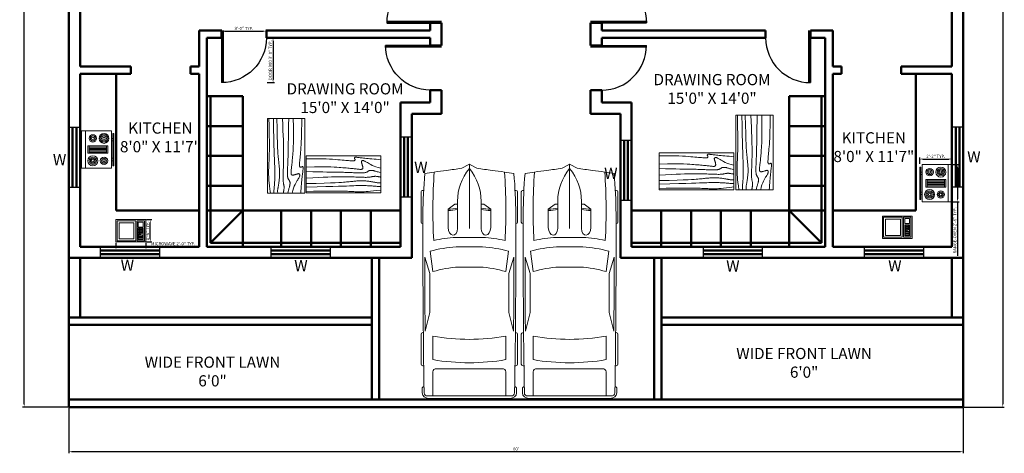
# Model space of a CAD drawing. Units: inches. Extents: x 2663 to 4539, y 2314 to 3111.
# Tile 1 of 4: x 2663 to 3456, y 2314 to 2663. Entities that reach past the tile are written whole.
import ezdxf

# ---------------------------------------------------------------- set-up
doc = ezdxf.new("R2010")
doc.units = ezdxf.units.IN
for name, color, linetype, lineweight in [('A-ANNO-DIMS', 2, 'Continuous', 18), ('A-ANNO-TEXT', 7, 'Continuous', 18), ('A-AREA-IDEN', 3, 'Continuous', 25), ('A-DOOR', 4, 'Continuous', 25), ('A-EQPM', 9, 'Continuous', 18), ('A-FURN', 8, 'Continuous', 18), ('A-GLAZ', 3, 'Continuous', 25), ('A-WALL', 7, 'Continuous', 50), ('C-PRKG', 9, 'Continuous', 18)]:
    doc.layers.add(name, color=color, linetype=linetype, lineweight=lineweight)
doc.styles.get("Standard").update_dxf_attribs({"font": 'arial.ttf'})
doc.dimstyles.new('ISO-25', dxfattribs={"dimtxt": 2.5, "dimasz": 2.5, "dimexe": 1.25, "dimexo": 0.625, "dimtad": 1, "dimdec": 0, "dimlunit": 3, "dimtxsty": 'Standard', "dimcen": 2.5, "dimadec": 0, "dimazin": 0, "dimtfac": 1, "dimtdec": 0, "dimtmove": 0, "dimatfit": 3, "dimfxl": 1, "dimarcsym": 0})

# ---------------------------------------------------------------- blocks, each defined once
blk = doc.blocks.new('Table - Rectangular Woodgrain 60 x 30 in.')
for p, q in [((0, 0), (0, -30)), ((60, 0), (0, 0)), ((60, -30), (60, 0)), ((0, -30), (60, -30))]:
    blk.add_line(p, q)
for points in [[(0, -2.4), (4.8155, -2.418), (9.0302, -2.4688), (12.709, -2.5477), (15.9167, -2.65), (18.7181, -2.7711), (21.1781, -2.9063), (23.3616, -3.0508), (25.3333, -3.2), (27.1477, -3.3495), (28.8172, -3.4958), (30.3437, -3.636), (31.7291, -3.7667), (32.9756, -3.8849), (34.0849, -3.9875), (35.059, -4.0714), (35.9, -4.1334), (36.6114, -4.1711), (37.2041, -4.1854), (37.6906, -4.1779), (38.0833, -4.15), (38.3948, -4.1034), (38.6375, -4.0396), (38.8239, -3.9602), (38.9666, -3.8667), (39.0764, -3.7608), (39.1573, -3.6448), (39.2116, -3.521), (39.2416, -3.3917), (39.2498, -3.2593), (39.2385, -3.1261), (39.21, -2.9944), (39.1666, -2.8667), (39.111, -2.7447), (39.0468, -2.6281), (38.978, -2.5163), (38.9083, -2.4083), (38.8418, -2.3035), (38.7823, -2.201), (38.7337, -2.1001), (38.7, -2), (38.6844, -1.9003), (38.6875, -1.8021), (38.7094, -1.707), (38.75, -1.6167), (38.8094, -1.5326), (38.8875, -1.4563), (38.9844, -1.3893), (39.1, -1.3333), (39.2351, -1.2896), (39.3937, -1.2583), (39.5804, -1.2396), (39.8, -1.2333), (40.057, -1.2396), (40.3562, -1.2583), (40.7023, -1.2896), (41.1, -1.3333), (41.5547, -1.3895), (42.0755, -1.4573), (42.6721, -1.5361), (43.3542, -1.625), (44.1316, -1.7233), (45.014, -1.8302), (46.0114, -1.9449), (47.1333, -2.0667), (48.3862, -2.1947), (49.7625, -2.3281), (51.2513, -2.4663), (52.8416, -2.6083), (54.5226, -2.7535), (56.2833, -2.9011), (58.1127, -3.0501), (60, -3.2)], [(0, -9.2), (6.5759, -9.0858), (11.9385, -9.0365), (16.2527, -9.0418), (19.6833, -9.0917), (22.3952, -9.1759), (24.5531, -9.2844), (26.322, -9.4069), (27.8666, -9.5333), (29.3241, -9.6553), (30.7203, -9.7719), (32.0532, -9.8837), (33.3208, -9.9917), (34.5213, -10.0965), (35.6526, -10.199), (36.7128, -10.2999), (37.7, -10.4), (38.6129, -10.4996), (39.4531, -10.5969), (40.223, -10.6895), (40.925, -10.775), (41.5613, -10.8512), (42.1344, -10.9156), (42.6465, -10.966), (43.1, -11), (43.4976, -11.0158), (43.8437, -11.0136), (44.143, -10.9942), (44.4, -10.9583), (44.6195, -10.9069), (44.8062, -10.8406), (44.9648, -10.7603), (45.1, -10.6667), (45.2155, -10.5598), (45.3114, -10.4365), (45.3871, -10.2929), (45.4416, -10.125), (45.4743, -9.929), (45.4844, -9.7011), (45.4709, -9.4371), (45.4333, -9.1333), (45.3716, -8.7883), (45.2896, -8.4104), (45.1919, -8.0107), (45.0833, -7.6), (44.9685, -7.1893), (44.8521, -6.7896), (44.7388, -6.4117), (44.6333, -6.0667), (44.54, -5.7628), (44.4614, -5.4979), (44.4001, -5.2675), (44.3583, -5.0667), (44.3384, -4.8909), (44.3427, -4.7354), (44.3736, -4.5956), (44.4333, -4.4667), (44.5236, -4.3453), (44.6427, -4.2333), (44.7884, -4.1339), (44.9583, -4.05), (45.1501, -3.9849), (45.3614, -3.9417), (45.59, -3.9234), (45.8333, -3.9333), (46.0915, -3.9749), (46.3734, -4.0531), (46.6906, -4.1736), (47.0542, -4.3417), (47.4756, -4.5629), (47.9661, -4.8427), (48.5372, -5.1866), (49.2, -5.6), (49.9676, -6.0844), (50.8594, -6.625), (51.8965, -7.2031), (53.1, -7.8), (54.491, -8.3969), (56.0906, -8.975), (57.9199, -9.5156), (60, -10)], [(0, -12.8), (5.1847, -12.9322), (9.6213, -13.0323), (13.3963, -13.1059), (16.5958, -13.1583), (19.3063, -13.1952), (21.614, -13.2219), (23.6054, -13.2439), (25.3666, -13.2667), (26.9728, -13.2947), (28.4531, -13.3281), (29.8256, -13.3663), (31.1083, -13.4083), (32.3191, -13.4535), (33.476, -13.501), (34.597, -13.5501), (35.7, -13.6), (36.7984, -13.6497), (37.8875, -13.6979), (38.9578, -13.743), (40, -13.7833), (41.0047, -13.8174), (41.9625, -13.8438), (42.864, -13.8607), (43.7, -13.8667), (44.4631, -13.8604), (45.1552, -13.8417), (45.7801, -13.8104), (46.3416, -13.7667), (46.8439, -13.7104), (47.2906, -13.6417), (47.6858, -13.5604), (48.0333, -13.4667), (48.3375, -13.3608), (48.6042, -13.2448), (48.8396, -13.121), (49.05, -12.9917), (49.2417, -12.8593), (49.4208, -12.7261), (49.5937, -12.5944), (49.7667, -12.4667), (49.9452, -12.3451), (50.1323, -12.2313), (50.3303, -12.1268), (50.5416, -12.0333), (50.7686, -11.9524), (51.0135, -11.8854), (51.2788, -11.8341), (51.5666, -11.8), (51.8785, -11.7843), (52.2116, -11.7865), (52.562, -11.8059), (52.926, -11.8417), (53.2998, -11.8931), (53.6795, -11.9594), (54.0614, -12.0397), (54.4416, -12.1333), (54.8223, -12.2401), (55.2293, -12.3625), (55.6942, -12.5037), (56.2489, -12.6667), (56.9251, -12.8547), (57.7545, -13.0708), (58.7689, -13.3182), (60, -13.6)], [(0, -18), (5.124, -17.7273), (9.6609, -17.5057), (13.6705, -17.3303), (17.2125, -17.1958), (20.3467, -17.0973), (23.1328, -17.0297), (25.6307, -16.9878), (27.9, -16.9667), (29.9928, -16.9617), (31.9302, -16.9703), (33.7254, -16.9907), (35.3917, -17.0208), (36.9423, -17.0588), (38.3906, -17.1026), (39.7499, -17.1503), (41.0333, -17.2), (42.2519, -17.2496), (43.4073, -17.2969), (44.4986, -17.3395), (45.525, -17.375), (46.4858, -17.4012), (47.3802, -17.4156), (48.2074, -17.416), (48.9667, -17.4), (49.6583, -17.3662), (50.2872, -17.3167), (50.8595, -17.2547), (51.3812, -17.1833), (51.8584, -17.1057), (52.2971, -17.025), (52.7034, -16.9443), (53.0833, -16.8667), (53.443, -16.7951), (53.789, -16.7313), (54.128, -16.6768), (54.4666, -16.6334), (54.8115, -16.6024), (55.1693, -16.5854), (55.5465, -16.5841), (55.95, -16.6), (56.3828, -16.6337), (56.8346, -16.6823), (57.2915, -16.7418), (57.7396, -16.8084), (58.165, -16.878), (58.5539, -16.9469), (58.8924, -17.0111), (59.1666, -17.0667), (59.3679, -17.1107), (59.5078, -17.1438), (59.6032, -17.1675), (59.6708, -17.1833), (59.7275, -17.193), (59.7901, -17.1979), (59.8753, -17.1998), (60, -17.2)], [(0, -22.4), (8.0098, -22.2501), (14.4094, -22.1011), (19.4168, -21.9535), (23.25, -21.8083), (26.1269, -21.6663), (28.2656, -21.5281), (29.884, -21.3947), (31.2, -21.2667), (32.3967, -21.1448), (33.5172, -21.0292), (34.5697, -20.9198), (35.5625, -20.8167), (36.5037, -20.7198), (37.4015, -20.6292), (38.2642, -20.5448), (39.1, -20.4667), (39.9164, -20.3951), (40.7187, -20.3313), (41.5117, -20.2768), (42.3, -20.2333), (43.0883, -20.2024), (43.8812, -20.1854), (44.6836, -20.1841), (45.5, -20.2), (46.3328, -20.234), (47.1747, -20.2844), (48.0163, -20.3488), (48.8479, -20.425), (49.66, -20.5106), (50.4429, -20.6031), (51.1872, -20.7004), (51.8833, -20.8), (52.5246, -20.8999), (53.1166, -20.9995), (53.6681, -21.0983), (54.1875, -21.1958), (54.6834, -21.2919), (55.1646, -21.3859), (55.6394, -21.4777), (56.1167, -21.5667), (56.6028, -21.6515), (57.0961, -21.7266), (57.5929, -21.7852), (58.0896, -21.8208), (58.5823, -21.8268), (59.0674, -21.7964), (59.5412, -21.723), (60, -21.6)], [(0, -25.2), (8.6355, -25.0504), (15.7026, -24.9031), (21.4049, -24.7606), (25.9458, -24.625), (29.529, -24.4988), (32.3578, -24.3844), (34.6359, -24.284), (36.5667, -24.2), (38.3213, -24.1341), (39.9417, -24.0854), (41.437, -24.0523), (42.8167, -24.0333), (44.0901, -24.0268), (45.2667, -24.0313), (46.3557, -24.0451), (47.3667, -24.0667), (48.309, -24.0947), (49.1928, -24.1287), (50.0284, -24.168), (50.826, -24.2125), (51.5959, -24.2617), (52.3483, -24.3151), (53.0935, -24.3725), (53.8417, -24.4334), (54.6009, -24.497), (55.3699, -24.561), (56.1454, -24.6226), (56.9239, -24.6792), (57.7021, -24.7279), (58.4764, -24.7662), (59.2435, -24.7911), (60, -24.8)], [(0, -28.8), (5.6867, -28.6681), (10.45, -28.5698), (14.407, -28.5012), (17.675, -28.4584), (20.3711, -28.4374), (22.6125, -28.4344), (24.5164, -28.4455), (26.2, -28.4667), (27.762, -28.4947), (29.2276, -28.5281), (30.6033, -28.5663), (31.8958, -28.6084), (33.1118, -28.6535), (34.2578, -28.7011), (35.3405, -28.7501), (36.3666, -28.8), (37.3443, -28.8497), (38.288, -28.8974), (39.2137, -28.9412), (40.1375, -28.9792), (41.0753, -29.0093), (42.0432, -29.0297), (43.0572, -29.0384), (44.1333, -29.0333), (45.2936, -29.0114), (46.5843, -28.9641), (48.0579, -28.8816), (49.7666, -28.7542), (51.7629, -28.5721), (54.0989, -28.3255), (56.8272, -28.0048), (60, -27.6)]]:
    blk.add_lwpolyline(points)
blk = doc.blocks.new('Range-Oven - 30 in top')
for p, q in [((0, -3), (30, -3)), ((12, -6), (18, -6)), ((13, -20), (13, -6)), ((14, -6), (14, -20)), ((15, -20), (15, -6)), ((16, -6), (16, -20)), ((17, -20), (17, -6)), ((18, -20), (12, -20)), ((6, -24), (6, -25)), ((8, -25), (8, -24)), ((22, -25), (22, -24)), ((24, -24), (24, -25))]:
    blk.add_line(p, q)
for points in [[(0, -24), (0, 0), (30, 0), (30, -24)], [(12, -21), (12, -5), (18, -5), (18, -21)], [(2, -26), (2, -25), (28, -25), (28, -26)]]:
    blk.add_lwpolyline(points, close=True)
for centre, radius in [((6, -9), 4), ((6, -9), 3), ((6, -9), 2), ((24, -9), 3), ((24, -9), 2), ((6, -18), 3), ((6, -9), 1), ((24, -18), 4), ((24, -18), 3), ((24, -9), 1), ((6, -18), 2), ((6, -18), 1), ((24, -18), 2), ((24, -18), 1)]:
    blk.add_circle(centre, radius)
blk = doc.blocks.new('Microwave')
for p, q in [((18, 10), (22, 10)), ((22, 9), (18, 9)), ((18, 8), (22, 8)), ((19, 7), (19, 11)), ((20, 11), (20, 7)), ((21, 7), (21, 11)), ((22, 7), (18, 7)), ((20, 6), (18, 6)), ((19, 6), (19, 7)), ((20, 7), (20, 6))]:
    blk.add_line(p, q)
for points in [[(0, 0), (0, 18), (24, 18), (24, 0)], [(1, 1), (1, 17), (16, 17), (16, 1)], [(17, 1), (17, 17), (23, 17), (23, 1)], [(18, 12), (18, 16), (22, 16), (22, 12)], [(2.5, 2.5), (2.5, 15.5), (14.5, 15.5), (14.5, 2.5)], [(18, 2), (18, 11), (22, 11), (22, 2)], [(18.5, 4.5), (18.5, 5.5), (21.5, 5.5), (21.5, 4.5)], [(18.5, 3), (18.5, 4), (21.5, 4), (21.5, 3)]]:
    blk.add_lwpolyline(points, close=True)
blk = doc.blocks.new('*D11')
at = {"layer": 'A-ANNO-DIMS', "color": 0, "lineweight": -2, "transparency": 16777216}
for p, q in [((3423.26, 3070.91), (3455.77, 3070.91)), ((3454.52, 3068.41), (3454.52, 2353.41)), ((3423.26, 2350.91), (3455.77, 2350.91))]:
    blk.add_line(p, q, dxfattribs=at)
at = {"layer": 'A-ANNO-DIMS', "color": 0, "transparency": 16777216}
for points in [[(3454.11, 3068.41), (3454.94, 3068.41), (3454.52, 3070.91)], [(3454.11, 2353.41), (3454.94, 2353.41), (3454.52, 2350.91)]]:
    blk.add_solid(points, dxfattribs=at)
at = {"layer": 'Defpoints', "color": 0, "transparency": 16777216}
for p in [(3422.63, 3070.91), (3422.63, 2350.91), (3454.52, 2350.91)]:
    blk.add_point(p, dxfattribs=at)
at = {"layer": 'A-ANNO-DIMS', "color": 0, "transparency": 16777216, "insert": (3452.62, 2710.91), "char_height": 2.5, "attachment_point": 5, "rotation": 90}
blk.add_mtext("60'", dxfattribs=at)
blk = doc.blocks.new('*U13')
for p, q in [((21.1, 37.41), (21.1, 36.83)), ((46.55, 38.89), (22.35, 38.89)), ((47.8, 37.39), (47.8, 37.41)), ((87.99, 31.87), (74.76, 35.92)), ((134.31, 35.6), (119.29, 31.78)), ((135.45, 37.07), (135.45, 37.41)), ((136.7, 38.89), (160.9, 38.89)), ((162.15, 37.41), (162.15, 36.77)), ((186.47, -33.5), (186.47, 33.5)), ((188.4, -32.76), (188.4, 32.76)), ((70.03, 31.54), (86.41, 29.35)), ((138.42, 29.35), (157.25, 29.35)), ((164.52, 26.39), (164.52, -26.39)), ((186.47, 29.35), (167.01, 29.35)), ((32.27, 11.63), (36.13, 17.17)), ((36.13, 17.17), (50.94, 17.17)), ((29.77, 9.51), (51.68, 9.51)), ((32.12, 9.51), (32.12, 11.15)), ((58.92, -10.77), (58.92, 10.77)), ((66.55, -10.53), (66.55, 10.53)), ((82.74, 8.5), (82.74, -8.5)), ((186.47, -10.53), (186.47, 10.53)), ((3.27, 6.13), (0.1, 0.41)), ((0, 0), (51.68, 0)), ((0.1, -0.41), (3.27, -6.13)), ((29.77, -9.51), (51.68, -9.51)), ((32.12, -9.51), (32.12, -11.15)), ((32.27, -11.63), (36.13, -17.17)), ((36.13, -17.17), (50.94, -17.17)), ((86.41, -29.35), (70.03, -31.54)), ((157.25, -29.35), (138.42, -29.35)), ((167.01, -29.35), (186.47, -29.35)), ((21.1, -37.41), (21.1, -36.83)), ((46.55, -38.89), (22.35, -38.89)), ((47.8, -37.39), (47.8, -37.41)), ((87.99, -31.87), (74.76, -35.92)), ((134.31, -35.6), (119.29, -31.78)), ((135.45, -37.07), (135.45, -37.41)), ((136.7, -38.89), (160.9, -38.89)), ((162.15, -37.41), (162.15, -36.77))]:
    blk.add_line(p, q)
for centre, major_axis, ratio, start_param, end_param in [((266.03, -27.52), (0, 313.31), 0.842304, 1.367076, 1.39176), ((41.19, -490.86), (0, 528.23), 0.842304, 0.00281, 0.075598), ((22.35, 37.41), (0, -1.48), 0.842304, 3.141593, 4.712389), ((64.48, -10555.62), (0, 10593.03), 0.842304, -0.013397, 0.002797), ((46.55, 37.41), (0, 1.48), 0.842304, -1.570796, 0), ((64.48, -10555.62), (0, -10591.55), 0.842304, 3.133765, 3.140441), ((95.79, -3666.35), (0, -3698.24), 0.842304, 3.134049, 3.144098), ((136.7, 37.41), (0, -1.48), 0.842304, 3.141593, 4.712389), ((160.9, 37.41), (0, 1.48), 0.842304, -1.570796, 0), ((180.63, 35.84), (0, 2.22), 0.842304, -0.013017, 1.249894), ((64.48, -10556.36), (0, 10595.31), 0.842304, -0.013397, -0.013017), ((183.98, 33.5), (0, -2.96), 0.842304, 1.570796, 3.128196), ((183.98, 32.76), (0, -5.25), 0.842304, 1.570796, 3.128196), ((259.18, -27.52), (0, -305.3), 0.842304, 4.528606, 4.561838), ((37.47, -593.96), (0, -623.33), 0.842304, 3.096046, 3.200911), ((134.4, 5.39), (0, -89.78), 0.842304, 4.449482, 4.652344), ((135.29, 5.39), (0, 81.77), 0.842304, 1.245306, 1.50788), ((149.6, 2.8), (0, -79.58), 0.842304, 4.372215, 4.640744), ((17.08, 0), (0, 147.02), 0.842304, 4.511394, 4.913384), ((35.91, 0), (0, 147.02), 0.842304, 4.511394, 4.913384), ((167.01, 26.39), (0, 2.96), 0.842304, 0, 1.570796), ((-204.49, 52.4), (0, -250.96), 0.842304, 1.385369, 1.434372), ((13.04, 17.01), (0, 27.42), 0.842304, 4.435146, 4.718221), ((14.2, 17.01), (0, 27.42), 0.842304, 4.435146, 4.718221), ((50.79, 13.34), (6.34, -0.36), 0.603834, -1.395552, 1.581315), ((29.77, -46.66), (0, 56.17), 0.842304, 0, 0.590319), ((32.75, 11.15), (0, 0.74), 0.842304, 0.879714, 1.570796), ((0.62, 0), (0, -0.74), 0.842304, 4.131459, 5.293319), ((-204.49, -52.4), (0, 250.96), 0.842304, -1.434372, -1.385369), ((29.77, 46.66), (0, 56.17), 0.842304, 2.551274, 3.141593), ((32.75, -11.15), (0, -0.74), 0.842304, 4.712389, 5.403472), ((13.04, -17.01), (0, -27.42), 0.842304, 1.564964, 1.848039), ((14.2, -17.01), (0, -27.42), 0.842304, 1.564964, 1.848039), ((134.4, -5.39), (0, -89.78), 0.842304, -1.510751, -1.307889), ((135.29, -5.39), (0, -81.77), 0.842304, -1.50788, -1.245306), ((149.6, -2.8), (0, -79.58), 0.842304, -1.499151, -1.230623), ((259.18, 27.52), (0, 305.3), 0.842304, 1.721348, 1.754579), ((266.03, 27.52), (0, 313.31), 0.842304, 1.749832, 1.774517), ((37.47, 593.96), (0, -623.33), 0.842304, -0.059319, 0.045547), ((167.01, -26.39), (0, -2.96), 0.842304, 4.712389, 6.283185), ((41.19, 490.86), (0, -528.23), 0.842304, -0.075598, -0.00281), ((22.35, -37.41), (0, 1.48), 0.842304, 1.570796, 3.141593), ((64.48, 10555.62), (0, 10593.03), 0.842304, 3.138796, 3.15499), ((46.55, -37.41), (0, -1.48), 0.842304, 0, 1.570796), ((64.48, 10555.62), (0, -10591.55), 0.842304, 0.001152, 0.007828), ((95.79, 3666.35), (0, -3698.24), 0.842304, -0.002505, 0.007544), ((136.7, -37.41), (0, -1.48), 0.842304, -1.570796, 0), ((160.9, -37.41), (0, 1.48), 0.842304, 3.141593, 4.712389), ((180.63, -35.84), (0, -2.22), 0.842304, -1.249894, 0.013017), ((64.48, 10556.36), (0, 10595.31), 0.842304, 3.15461, 3.15499), ((183.98, -33.5), (0, 2.96), 0.842304, 3.15499, 4.712389), ((183.98, -32.76), (0, -5.25), 0.842304, 0.013397, 1.570796)]:
    blk.add_ellipse(centre, major_axis=major_axis, ratio=ratio, start_param=start_param, end_param=end_param)
at = {"extrusion": (0, 0, -1)}
blk.add_ellipse((50.79, -13.34), major_axis=(6.34, 0.36), ratio=0.603834, start_param=-1.395552, end_param=1.581315, dxfattribs=at)
blk = doc.blocks.new('*D18')
at = {"layer": 'A-ANNO-DIMS', "color": 0, "lineweight": -2, "transparency": 16777216}
for p, q in [((2702.63, 2350.29), (2702.63, 2313.66)), ((3422.63, 2350.29), (3422.63, 2313.66)), ((3420.13, 2314.91), (2705.13, 2314.91))]:
    blk.add_line(p, q, dxfattribs=at)
at = {"layer": 'A-ANNO-DIMS', "color": 0, "transparency": 16777216}
for points in [[(2705.13, 2315.33), (2705.13, 2314.5), (2702.63, 2314.91)], [(3420.13, 2315.33), (3420.13, 2314.5), (3422.63, 2314.91)]]:
    blk.add_solid(points, dxfattribs=at)
at = {"layer": 'Defpoints', "color": 0, "transparency": 16777216}
for p in [(2702.63, 2350.91), (3422.63, 2350.91), (2702.63, 2314.91)]:
    blk.add_point(p, dxfattribs=at)
at = {"layer": 'A-ANNO-DIMS', "color": 0, "transparency": 16777216, "insert": (3062.63, 2316.82), "char_height": 2.5, "attachment_point": 5}
blk.add_mtext("60'", dxfattribs=at)
blk = doc.blocks.new('*D19')
at = {"layer": 'A-ANNO-DIMS', "color": 0, "lineweight": -2, "transparency": 16777216}
for p, q in [((2702.01, 3070.91), (2665.38, 3070.91)), ((2666.63, 2353.41), (2666.63, 3068.41)), ((2702.01, 2350.91), (2665.38, 2350.91))]:
    blk.add_line(p, q, dxfattribs=at)
at = {"layer": 'A-ANNO-DIMS', "color": 0, "transparency": 16777216}
for points in [[(2666.21, 3068.41), (2667.05, 3068.41), (2666.63, 3070.91)], [(2666.21, 2353.41), (2667.05, 2353.41), (2666.63, 2350.91)]]:
    blk.add_solid(points, dxfattribs=at)
at = {"layer": 'Defpoints', "color": 0, "transparency": 16777216}
for p in [(2666.63, 3070.91), (2702.63, 3070.91), (2702.63, 2350.91)]:
    blk.add_point(p, dxfattribs=at)
at = {"layer": 'A-ANNO-DIMS', "color": 0, "transparency": 16777216, "insert": (2664.73, 2710.91), "char_height": 2.5, "attachment_point": 5, "rotation": 90}
blk.add_mtext("60'", dxfattribs=at)
blk = doc.blocks.new('WIN-1200')
for p, q in [((0, 48), (0, 0)), ((9, 48), (0, 48)), ((0, 48), (0, 48)), ((9, 0), (9, 48)), ((0, 0), (9, 0))]:
    blk.add_line(p, q)
blk = doc.blocks.new('DOOR-900')
blk.add_line((3071.63, 2949.91), (3071.63, 2985.91))
blk.add_arc((3071.63, 2949.91), 36, 0, 90)
blk = doc.blocks.new('*D28')
at = {"layer": 'A-ANNO-DIMS', "color": 0, "lineweight": -2, "transparency": 16777216}
for p, q in [((2862.26, 2647.91), (2868.28, 2647.91)), ((2867.03, 2645.41), (2867.03, 2614.41)), ((2862.26, 2611.91), (2868.28, 2611.91))]:
    blk.add_line(p, q, dxfattribs=at)
at = {"layer": 'A-ANNO-DIMS', "color": 0, "transparency": 16777216}
for points in [[(2866.61, 2645.41), (2867.45, 2645.41), (2867.03, 2647.91)], [(2866.61, 2614.41), (2867.45, 2614.41), (2867.03, 2611.91)]]:
    blk.add_solid(points, dxfattribs=at)
at = {"layer": 'Defpoints', "color": 0, "transparency": 16777216}
for p in [(2861.63, 2647.91), (2861.63, 2611.91), (2867.03, 2611.91)]:
    blk.add_point(p, dxfattribs=at)
at = {"layer": 'A-ANNO-DIMS', "color": 0, "transparency": 16777216, "insert": (2865.11, 2629.91), "char_height": 2.5, "attachment_point": 5, "rotation": 90}
blk.add_mtext('DOOR 900 3\'-0" TYP.', dxfattribs=at)
blk = doc.blocks.new('*D29')
at = {"layer": 'A-ANNO-DIMS', "color": 0, "lineweight": -2, "transparency": 16777216}
for p, q in [((2825.63, 2648.54), (2825.63, 2654.56)), ((2828.13, 2653.31), (2859.13, 2653.31)), ((2861.63, 2648.54), (2861.63, 2654.56))]:
    blk.add_line(p, q, dxfattribs=at)
at = {"layer": 'A-ANNO-DIMS', "color": 0, "transparency": 16777216}
for points in [[(2828.13, 2653.73), (2828.13, 2652.9), (2825.63, 2653.31)], [(2859.13, 2653.73), (2859.13, 2652.9), (2861.63, 2653.31)]]:
    blk.add_solid(points, dxfattribs=at)
at = {"layer": 'Defpoints', "color": 0, "transparency": 16777216}
for p in [(2825.63, 2647.91), (2861.63, 2653.31), (2861.63, 2647.91)]:
    blk.add_point(p, dxfattribs=at)
at = {"layer": 'A-ANNO-DIMS', "color": 0, "transparency": 16777216, "insert": (2843.63, 2655.22), "char_height": 2.5, "attachment_point": 5}
blk.add_mtext('3\'-0" TYP.', dxfattribs=at)
blk = doc.blocks.new('*D46')
at = {"layer": 'A-ANNO-DIMS', "color": 0, "lineweight": -2, "transparency": 16777216}
for p, q in [((3414.26, 2545.91), (3419.38, 2545.91)), ((3418.13, 2543.41), (3418.13, 2518.41)), ((3414.26, 2515.91), (3419.38, 2515.91)), ((3418.13, 2515.91), (3418.13, 2472.6))]:
    blk.add_line(p, q, dxfattribs=at)
at = {"layer": 'A-ANNO-DIMS', "color": 0, "transparency": 16777216}
for points in [[(3417.71, 2543.41), (3418.55, 2543.41), (3418.13, 2545.91)], [(3417.71, 2518.41), (3418.55, 2518.41), (3418.13, 2515.91)]]:
    blk.add_solid(points, dxfattribs=at)
at = {"layer": 'Defpoints', "color": 0, "transparency": 16777216}
for p in [(3413.63, 2545.91), (3413.63, 2515.91), (3418.13, 2515.91)]:
    blk.add_point(p, dxfattribs=at)
at = {"layer": 'A-ANNO-DIMS', "color": 0, "transparency": 16777216, "insert": (3416.21, 2493), "char_height": 2.5, "attachment_point": 5, "rotation": 90}
blk.add_mtext('RANGE-OVEN 2\'-6" TYP.', dxfattribs=at)
blk = doc.blocks.new('*D47')
at = {"layer": 'A-ANNO-DIMS', "color": 0, "lineweight": -2, "transparency": 16777216}
for p, q in [((3387.63, 2546.53), (3387.63, 2551.66)), ((3390.13, 2550.41), (3411.13, 2550.41)), ((3413.63, 2546.53), (3413.63, 2551.66))]:
    blk.add_line(p, q, dxfattribs=at)
at = {"layer": 'A-ANNO-DIMS', "color": 0, "transparency": 16777216}
for points in [[(3390.13, 2550.82), (3390.13, 2549.99), (3387.63, 2550.41)], [(3411.13, 2550.82), (3411.13, 2549.99), (3413.63, 2550.41)]]:
    blk.add_solid(points, dxfattribs=at)
at = {"layer": 'Defpoints', "color": 0, "transparency": 16777216}
for p in [(3387.63, 2545.91), (3413.63, 2550.41), (3413.63, 2545.91)]:
    blk.add_point(p, dxfattribs=at)
at = {"layer": 'A-ANNO-DIMS', "color": 0, "transparency": 16777216, "insert": (3400.63, 2552.29), "char_height": 2.5, "attachment_point": 5}
blk.add_mtext('2\'-2" TYP.', dxfattribs=at)
blk = doc.blocks.new('*D48')
at = {"layer": 'A-ANNO-DIMS', "color": 0, "lineweight": -2, "transparency": 16777216}
for p, q in [((2740.52, 2483.06), (2740.52, 2478.84)), ((2764.52, 2483.06), (2764.52, 2478.84)), ((2743.02, 2480.09), (2762.02, 2480.09)), ((2764.52, 2480.09), (2806.29, 2480.09))]:
    blk.add_line(p, q, dxfattribs=at)
at = {"layer": 'A-ANNO-DIMS', "color": 0, "transparency": 16777216}
for points in [[(2743.02, 2480.51), (2743.02, 2479.67), (2740.52, 2480.09)], [(2762.02, 2480.51), (2762.02, 2479.67), (2764.52, 2480.09)]]:
    blk.add_solid(points, dxfattribs=at)
at = {"layer": 'Defpoints', "color": 0, "transparency": 16777216}
for p in [(2740.52, 2483.69), (2764.52, 2483.69), (2764.52, 2480.09)]:
    blk.add_point(p, dxfattribs=at)
at = {"layer": 'A-ANNO-DIMS', "color": 0, "transparency": 16777216, "insert": (2786.66, 2482.01), "char_height": 2.5, "attachment_point": 5}
blk.add_mtext('MICROWAVE 2\'-0" TYP.', dxfattribs=at)
blk = doc.blocks.new('*D49')
at = {"layer": 'A-ANNO-DIMS', "color": 0, "lineweight": -2, "transparency": 16777216}
for p, q in [((2765.15, 2501.69), (2769.37, 2501.69)), ((2768.12, 2486.19), (2768.12, 2499.19)), ((2765.15, 2483.69), (2769.37, 2483.69))]:
    blk.add_line(p, q, dxfattribs=at)
at = {"layer": 'A-ANNO-DIMS', "color": 0, "transparency": 16777216}
for points in [[(2767.7, 2499.19), (2768.54, 2499.19), (2768.12, 2501.69)], [(2767.7, 2486.19), (2768.54, 2486.19), (2768.12, 2483.69)]]:
    blk.add_solid(points, dxfattribs=at)
at = {"layer": 'Defpoints', "color": 0, "transparency": 16777216}
for p in [(2764.52, 2501.69), (2768.12, 2501.69), (2764.52, 2483.69)]:
    blk.add_point(p, dxfattribs=at)
at = {"layer": 'A-ANNO-DIMS', "color": 0, "transparency": 16777216, "insert": (2766.22, 2492.69), "char_height": 2.5, "attachment_point": 5, "rotation": 90}
blk.add_mtext('1\'-6" TYP.', dxfattribs=at)

msp = doc.modelspace()

# ---------------------------------------------------------------- linework, layer by layer
at = {"layer": 'A-DOOR'}
msp.add_arc((2993.63, 2660.91), 35, 90, 181.63725, dxfattribs=at)
at = {"layer": 'A-WALL'}
for p, q in [((2702.63, 2350.91), (2702.63, 3070.91)), ((3422.63, 3070.91), (3422.63, 2350.91)), ((2711.63, 2624.91), (2711.63, 3061.91)), ((3413.63, 2789.91), (3413.63, 2624.91)), ((2993.63, 2660.91), (2958.63, 2660.91)), ((2993.63, 2659.91), (2958.64, 2659.91)), ((2993.63, 2660.91), (3002.63, 2660.91)), ((2993.63, 2653.91), (2993.63, 2659.91)), ((2993.63, 2659.91), (3002.63, 2659.91)), ((2993.63, 2659.91), (2993.63, 2653.91)), ((3002.63, 2659.91), (3002.63, 2641.91)), ((3002.63, 2659.91), (3002.63, 2653.91)), ((3131.63, 2660.91), (3122.63, 2660.91)), ((3131.63, 2659.91), (3122.63, 2659.91)), ((3122.63, 2659.91), (3122.63, 2653.91)), ((3122.63, 2659.91), (3122.63, 2641.91)), ((3131.63, 2660.91), (3167.63, 2660.91)), ((3131.63, 2653.91), (3131.63, 2659.91)), ((3131.63, 2659.91), (3131.63, 2653.91)), ((2807.63, 2653.91), (2825.63, 2653.91)), ((2807.63, 2624.91), (2807.63, 2653.91)), ((2813.63, 2647.91), (2825.63, 2647.91)), ((2813.63, 2624.91), (2813.63, 2647.91)), ((2813.63, 2647.91), (2825.63, 2647.91)), ((2825.63, 2647.91), (2825.63, 2653.91)), ((2826.63, 2647.91), (2826.63, 2653.91)), ((2826.63, 2647.91), (2826.63, 2611.91)), ((2861.63, 2653.91), (2861.63, 2647.91)), ((2861.63, 2653.91), (2993.63, 2653.91)), ((2861.63, 2647.91), (2993.63, 2647.91)), ((2993.63, 2647.91), (2993.63, 2641.91)), ((2993.63, 2647.91), (2993.63, 2641.91)), ((3002.63, 2647.91), (3002.63, 2641.91)), ((3122.63, 2647.91), (3122.63, 2641.91)), ((3131.63, 2653.91), (3263.63, 2653.91)), ((3131.63, 2647.91), (3263.63, 2647.91)), ((3131.63, 2647.91), (3131.63, 2641.91)), ((3131.63, 2647.91), (3131.63, 2641.91)), ((3263.63, 2653.91), (3263.63, 2647.91)), ((3298.63, 2647.91), (3298.63, 2653.91)), ((3298.63, 2647.91), (3298.63, 2611.91)), ((3299.63, 2647.91), (3299.63, 2653.91)), ((3299.63, 2653.91), (3317.63, 2653.91)), ((3311.63, 2647.91), (3299.63, 2647.91)), ((3299.63, 2647.91), (3311.63, 2647.91)), ((3311.63, 2624.91), (3311.63, 2647.91)), ((3317.63, 2624.91), (3317.63, 2653.91)), ((2993.63, 2640.91), (2957.63, 2640.91)), ((2993.63, 2641.91), (3002.63, 2641.91)), ((2993.63, 2640.91), (3002.63, 2640.91)), ((3131.63, 2641.91), (3122.63, 2641.91)), ((3131.63, 2640.91), (3122.63, 2640.91)), ((3131.63, 2640.91), (3167.63, 2640.91)), ((2711.63, 2624.91), (2752.63, 2624.91)), ((2752.63, 2618.91), (2752.63, 2624.91)), ((2800.63, 2624.91), (2800.63, 2618.91)), ((2800.63, 2624.91), (2807.63, 2624.91)), ((2813.63, 2479.91), (2813.63, 2624.91)), ((3311.63, 2624.91), (3311.63, 2479.91)), ((3317.63, 2624.91), (3324.63, 2624.91)), ((3324.63, 2618.91), (3324.63, 2624.91)), ((3401.63, 2624.91), (3372.63, 2624.91)), ((3372.63, 2624.91), (3372.63, 2618.91)), ((3372.63, 2624.91), (3413.63, 2624.91)), ((3413.63, 2624.91), (3401.63, 2624.91)), ((2711.63, 2618.91), (2752.63, 2618.91)), ((2711.63, 2479.91), (2711.63, 2618.91)), ((2711.63, 2618.91), (2723.63, 2618.91)), ((2723.63, 2618.91), (2752.63, 2618.91)), ((2740.63, 2508.91), (2740.63, 2618.91)), ((2800.63, 2618.91), (2807.63, 2618.91)), ((2807.63, 2479.91), (2807.63, 2618.91)), ((3317.63, 2618.91), (3317.63, 2479.91)), ((3317.63, 2618.91), (3324.63, 2618.91)), ((3372.63, 2618.91), (3413.63, 2618.91)), ((3384.63, 2618.91), (3384.63, 2508.91)), ((3413.63, 2618.91), (3413.63, 2479.91)), ((2813.63, 2600.93), (2842.63, 2600.93)), ((2816.63, 2482.91), (2816.63, 2600.93)), ((2842.63, 2508.91), (2842.63, 2600.93)), ((2993.63, 2605.91), (2993.63, 2595.91)), ((3002.63, 2605.91), (2993.63, 2605.91)), ((3002.63, 2605.91), (3002.63, 2586.91)), ((3122.63, 2605.91), (3122.63, 2586.91)), ((3122.63, 2605.91), (3131.63, 2605.91)), ((3131.63, 2605.91), (3131.63, 2595.91)), ((3282.63, 2600.93), (3282.63, 2508.91)), ((3282.63, 2600.93), (3311.63, 2600.93)), ((3308.63, 2600.93), (3308.63, 2482.91)), ((2969.63, 2479.91), (2969.63, 2595.91)), ((2969.63, 2595.91), (2993.63, 2595.91)), ((3131.63, 2595.91), (3155.63, 2595.91)), ((3155.63, 2595.91), (3155.63, 2479.91)), ((2978.63, 2479.91), (2978.63, 2586.91)), ((2978.63, 2586.91), (2993.63, 2586.91)), ((2993.63, 2586.91), (3002.63, 2586.91)), ((3131.63, 2586.91), (3122.63, 2586.91)), ((3131.63, 2586.91), (3146.63, 2586.91)), ((3146.63, 2586.91), (3146.63, 2479.91)), ((2813.63, 2576.93), (2842.63, 2576.93)), ((3282.63, 2576.93), (3311.63, 2576.93)), ((2705.63, 2575.69), (2705.63, 2527.69)), ((2708.63, 2527.69), (2708.63, 2575.69)), ((3416.63, 2576.05), (3416.63, 2528.05)), ((3419.63, 2528.05), (3419.63, 2576.05)), ((2972.63, 2567.99), (2972.63, 2519.99)), ((2975.63, 2519.99), (2975.63, 2567.99)), ((3149.63, 2565.35), (3149.63, 2517.35)), ((3152.63, 2517.35), (3152.63, 2565.35)), ((2813.63, 2552.93), (2842.63, 2552.93)), ((3282.63, 2552.93), (3311.63, 2552.93)), ((2813.63, 2528.93), (2842.63, 2528.93)), ((3282.63, 2528.93), (3311.63, 2528.93)), ((2740.63, 2508.91), (2807.63, 2508.91)), ((2842.63, 2508.91), (2813.63, 2508.91)), ((2813.63, 2508.91), (2842.63, 2508.91)), ((2842.63, 2508.91), (2816.63, 2482.91)), ((2842.63, 2508.91), (2969.63, 2508.91)), ((2842.63, 2508.91), (2842.63, 2479.91)), ((2873.63, 2479.91), (2873.63, 2508.91)), ((2897.63, 2479.91), (2897.63, 2508.91)), ((2921.63, 2479.91), (2921.63, 2508.91)), ((2945.63, 2479.91), (2945.63, 2508.91)), ((3155.63, 2508.91), (3282.63, 2508.91)), ((3179.63, 2508.91), (3179.63, 2479.91)), ((3203.63, 2508.91), (3203.63, 2479.91)), ((3227.63, 2508.91), (3227.63, 2479.91)), ((3251.63, 2508.91), (3251.63, 2479.91)), ((3282.63, 2508.91), (3311.63, 2508.91)), ((3311.63, 2508.91), (3282.63, 2508.91)), ((3282.63, 2508.91), (3282.63, 2479.91)), ((3282.63, 2508.91), (3308.63, 2482.91)), ((3317.63, 2508.91), (3384.63, 2508.91)), ((2816.63, 2482.91), (2969.63, 2482.91)), ((3155.63, 2482.91), (3308.63, 2482.91)), ((2711.63, 2479.91), (2807.63, 2479.91)), ((2775.81, 2476.91), (2727.81, 2476.91)), ((2727.81, 2473.91), (2775.81, 2473.91)), ((2813.63, 2479.91), (2969.63, 2479.91)), ((2913.28, 2476.91), (2865.28, 2476.91)), ((2865.28, 2473.91), (2913.28, 2473.91)), ((2978.63, 2479.91), (2978.63, 2470.91)), ((3146.63, 2479.91), (3146.63, 2470.91)), ((3155.63, 2479.91), (3311.63, 2479.91)), ((3261.2, 2476.91), (3213.2, 2476.91)), ((3213.2, 2473.91), (3261.2, 2473.91)), ((3317.63, 2479.91), (3413.63, 2479.91)), ((3390.85, 2476.91), (3342.85, 2476.91)), ((3342.85, 2473.91), (3390.85, 2473.91)), ((2711.63, 2470.91), (2702.63, 2470.91)), ((2711.63, 2422.91), (2711.63, 2470.91)), ((2711.63, 2470.91), (2807.63, 2470.91)), ((2807.63, 2470.91), (2813.63, 2470.91)), ((2813.63, 2470.91), (2969.63, 2470.91)), ((2946.43, 2470.91), (2946.43, 2356.91)), ((2952.43, 2470.91), (2952.43, 2356.91)), ((2969.63, 2470.91), (2975.63, 2470.91)), ((2975.63, 2470.91), (2978.63, 2470.91)), ((3149.63, 2470.91), (3146.63, 2470.91)), ((3155.63, 2470.91), (3149.63, 2470.91)), ((3155.63, 2470.91), (3311.63, 2470.91)), ((3173.89, 2470.91), (3173.89, 2356.91)), ((3179.89, 2470.91), (3179.89, 2356.91)), ((3317.63, 2470.91), (3311.63, 2470.91)), ((3317.63, 2470.91), (3413.63, 2470.91)), ((3422.63, 2470.91), (3353.61, 2470.91)), ((3413.63, 2470.91), (3413.63, 2422.91)), ((3413.63, 2470.91), (3422.63, 2470.91)), ((2946.43, 2422.91), (2702.63, 2422.91)), ((3422.63, 2422.91), (3179.89, 2422.91)), ((2946.43, 2416.91), (2702.63, 2416.91)), ((3422.63, 2416.91), (3179.89, 2416.91)), ((3422.63, 2356.91), (2702.63, 2356.91)), ((3422.63, 2350.91), (2702.63, 2350.91))]:
    msp.add_line(p, q, dxfattribs=at)

# ---------------------------------------------------------------- block references
at = {"layer": 'A-DOOR', "extrusion": (0, 0, -1), "zscale": -1}
for p, rotation in [((-181.72, -411.72), 90.0000000000011), ((246, 5597.83), 180), ((-5943.55, 5713.55), 270.0000000000021)]:
    msp.add_blockref('DOOR-900', p, dxfattribs=dict(at, rotation=rotation))
at = {"layer": 'A-DOOR'}
for p, rotation in [((6371.26, 5597.83), 180), ((181.72, 5713.55), 270.0000000000014)]:
    msp.add_blockref('DOOR-900', p, dxfattribs=dict(at, rotation=rotation))
at = {"layer": 'A-EQPM'}
for p, rotation in [((2712.91, 2543.03), 90), ((3413.63, 2545.91), 270)]:
    msp.add_blockref('Range-Oven - 30 in top', p, dxfattribs=dict(at, rotation=rotation))
for p in [(2740.52, 2483.69), (3357.57, 2486.53)]:
    msp.add_blockref('Microwave', p, dxfattribs=at)
at = {"layer": 'A-FURN', "rotation": 270}
for p in [(3269.65, 2585.69), (2892.49, 2583.02)]:
    msp.add_blockref('Table - Rectangular Woodgrain 60 x 30 in.', p, dxfattribs=at)
at = {"layer": 'A-FURN'}
for p in [(2893.8, 2553.12), (3177.92, 2555.54)]:
    msp.add_blockref('Table - Rectangular Woodgrain 60 x 30 in.', p, dxfattribs=at)
at = {"layer": 'A-GLAZ'}
for p in [(2702.63, 2527.7), (3413.63, 2528.05), (2969.63, 2519.99), (3146.63, 2517.35)]:
    msp.add_blockref('WIN-1200', p, dxfattribs=at)
for p, rotation in [((2775.81, 2470.91), 89.9999999999986), ((2913.27, 2470.91), 89.99999999999825), ((3261.2, 2470.91), 89.9999999999977), ((3390.85, 2470.91), 89.99999999999704)]:
    msp.add_blockref('WIN-1200', p, dxfattribs=dict(at, rotation=rotation))
at = {"layer": 'C-PRKG', "rotation": 270}
for p in [(3025.06, 2546.27), (3105.79, 2546.27)]:
    msp.add_blockref('*U13', p, dxfattribs=at)

# ---------------------------------------------------------------- texts
at = {"layer": 'A-ANNO-TEXT', "char_height": 9, "attachment_point": 1}
for insert in [(2644.41, 2554.49), (3380.54, 2556.71), (2935.29, 2548.29), (3088.26, 2543.39), (2698.98, 2469.51), (2838.73, 2469.2), (3186.5, 2468.9), (3316.92, 2469)]:
    msp.add_mtext_dynamic_manual_height_columns('\\pxqc;W', width=101.4958, gutter_width=12.5, heights=[0], dxfattribs=dict(at, insert=insert))
at = {"layer": 'A-AREA-IDEN', "char_height": 9, "attachment_point": 1}
for s, width, insert in [('\\pxqc;DRAWING ROOM\\P15\'0" X 14\'0"', 107.0744, (3166.9, 2618.85)), ('\\pxqc;DRAWING ROOM\\P15\'0" X 14\'0"', 107.0744, (2871.48, 2611.42)), ('\\pxqc;KITCHEN\\P8\'0" X 11\'7"', 107.0744, (2722.75, 2579.85)), ('\\pxqc;KITCHEN\\P8\'0" X 11\'7"', 107.0744, (3297.2, 2571.98)), ('\\pxqc;WIDE FRONT LAWN\\P6\'0"', 201.8325, (3193.68, 2398.46)), ('\\pxqc;WIDE FRONT LAWN\\P6\'0"', 201.8325, (2717.36, 2391.48))]:
    msp.add_mtext_dynamic_manual_height_columns(s, width=width, gutter_width=12.5, heights=[0], dxfattribs=dict(at, insert=insert))

# ---------------------------------------------------------------- dimensions: what is measured, and where the dimension line sits
at = {"layer": 'A-ANNO-DIMS'}
for base, p1, p2, picture, middle in [((2666.63, 3070.91), (2702.63, 2350.91), (2702.63, 3070.91), '*D19', (2664.73, 2710.91)), ((3454.52, 2350.91), (3422.63, 3070.91), (3422.63, 2350.91), '*D11', (3452.62, 2710.91))]:
    dim = msp.add_linear_dim(base=base, p1=p1, p2=p2, angle=90, dimstyle='ISO-25', override={"dimclrd": 0, "dimclre": 0, "dimclrt": 0}, dxfattribs=at)
    dim.commit()
    dim.dimension.update_dxf_attribs({"geometry": picture, "text_midpoint": middle})
for base, p1, p2, text, picture, middle in [((2861.63, 2653.31), (2825.63, 2647.91), (2861.63, 2647.91), '<> TYP.', '*D29', (2843.63, 2655.22)), ((3413.63, 2550.41), (3387.63, 2545.91), (3413.63, 2545.91), '<> TYP.', '*D47', (3400.63, 2552.29)), ((2764.52, 2480.09), (2740.52, 2483.69), (2764.52, 2483.69), 'MICROWAVE <> TYP.', '*D48', (2786.66, 2482.01))]:
    dim = msp.add_linear_dim(base=base, p1=p1, p2=p2, text=text, dimstyle='ISO-25', override={"dimdec": 1, "dimrnd": 0, "dimzin": 1, "dimlunit": 4, "dimfrac": 2}, dxfattribs=at)
    dim.commit()
    dim.dimension.update_dxf_attribs({"geometry": picture, "text_midpoint": middle})
for base, p1, p2, angle, text, picture, middle in [((2867.03, 2611.91), (2861.63, 2647.91), (2861.63, 2611.91), 270, 'DOOR 900 <> TYP.', '*D28', (2865.11, 2629.91)), ((3418.13, 2515.91), (3413.63, 2545.91), (3413.63, 2515.91), 270, 'RANGE-OVEN <> TYP.', '*D46', (3416.21, 2493)), ((2768.12, 2501.69), (2764.52, 2483.69), (2764.52, 2501.69), 90, '<> TYP.', '*D49', (2766.22, 2492.69))]:
    dim = msp.add_linear_dim(base=base, p1=p1, p2=p2, angle=angle, text=text, dimstyle='ISO-25', override={"dimdec": 1, "dimrnd": 0, "dimzin": 1, "dimlunit": 4, "dimfrac": 2}, dxfattribs=at)
    dim.commit()
    dim.dimension.update_dxf_attribs({"geometry": picture, "text_midpoint": middle})
dim = msp.add_linear_dim(base=(2702.63, 2314.91), p1=(3422.63, 2350.91), p2=(2702.63, 2350.91), dimstyle='ISO-25', override={"dimclrd": 0, "dimclre": 0, "dimclrt": 0}, dxfattribs=at)
dim.commit()
dim.dimension.update_dxf_attribs({"geometry": '*D18', "text_midpoint": (3062.63, 2316.82)})

doc.saveas('drawing.dxf')
